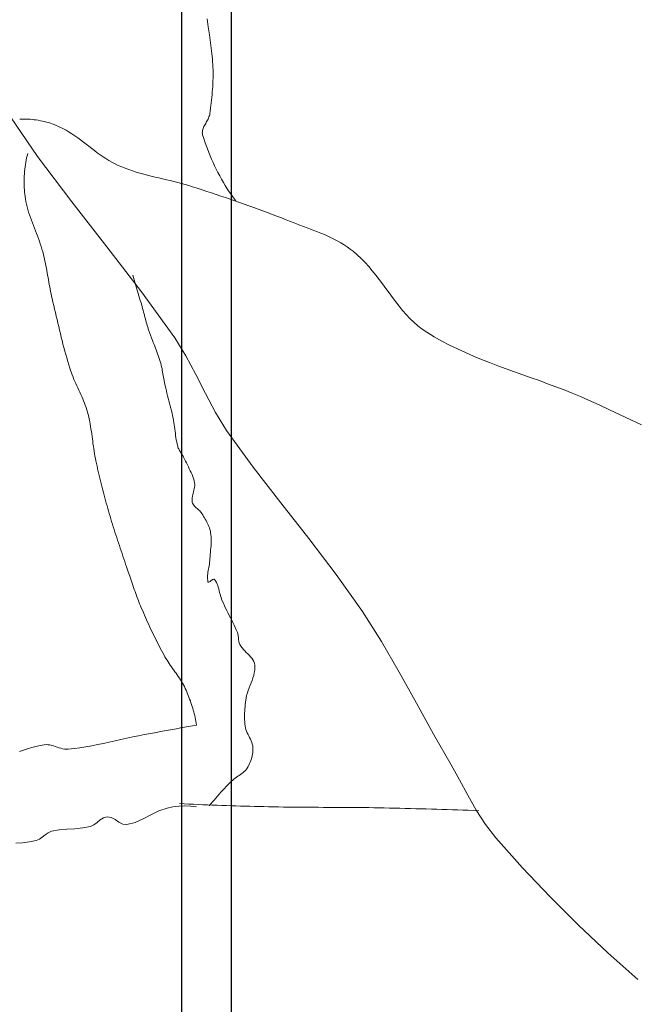
# Model space of a CAD drawing. Units: inches. Extents: x 2656 to 9931, y 1941 to 3068.
# Tile 8 of 46: x 2773 to 2792, y 2502 to 2533. Entities that reach past the tile are written whole.
import ezdxf

# ---------------------------------------------------------------- set-up
doc = ezdxf.new("R2010")
doc.units = ezdxf.units.IN
doc.layers.add('A-ANNO-DIMS', color=2, linetype='Continuous', lineweight=18)
doc.layers.add('A-FURN', color=8, linetype='Continuous', lineweight=13)
doc.styles.get("Standard").update_dxf_attribs({"font": 'arial.ttf'})
doc.dimstyles.new('ISO-25', dxfattribs={"dimtxt": 6, "dimasz": 2.5, "dimexe": 1.25, "dimexo": 0.625, "dimtad": 1, "dimdec": 0, "dimlunit": 3, "dimtxsty": 'Standard', "dimcen": 2.5, "dimadec": 0, "dimazin": 0, "dimtfac": 1, "dimtdec": 0, "dimtmove": 0, "dimatfit": 3, "dimfxl": 1, "dimarcsym": 0})

# ---------------------------------------------------------------- blocks, each defined once
blk = doc.blocks.new('BED-DOUBLE')
for p, q in [((24.978, 30.142), (25.017, 29.893)), ((25.017, 29.893), (25.054, 29.644)), ((25.054, 29.644), (25.087, 29.395)), ((25.087, 29.395), (25.118, 29.145)), ((25.118, 29.145), (25.146, 28.894)), ((25.146, 28.894), (25.153, 28.81)), ((25.153, 28.81), (25.159, 28.725)), ((25.159, 28.725), (25.164, 28.64)), ((25.164, 28.64), (25.166, 28.554)), ((25.166, 28.554), (25.168, 28.469)), ((25.163, 28.213), (25.16, 28.128)), ((25.166, 28.299), (25.163, 28.213)), ((25.168, 28.384), (25.166, 28.299)), ((25.168, 28.469), (25.168, 28.384)), ((25.149, 27.957), (25.142, 27.872)), ((25.155, 28.042), (25.149, 27.957)), ((25.16, 28.128), (25.155, 28.042)), ((25.118, 27.616), (25.108, 27.531)), ((25.127, 27.701), (25.118, 27.616)), ((25.135, 27.787), (25.127, 27.701)), ((25.142, 27.872), (25.135, 27.787)), ((18.699, 27.32), (19.702, 25.863)), ((25.078, 27.276), (25.067, 27.192)), ((25.088, 27.361), (25.078, 27.276)), ((25.098, 27.446), (25.088, 27.361)), ((25.108, 27.531), (25.098, 27.446)), ((19.217, 27.024), (19.153, 27.022)), ((19.28, 27.025), (19.217, 27.024)), ((19.344, 27.025), (19.28, 27.025)), ((19.408, 27.022), (19.344, 27.025)), ((19.472, 27.018), (19.408, 27.022)), ((19.535, 27.013), (19.472, 27.018)), ((19.599, 27.006), (19.535, 27.013)), ((19.663, 26.997), (19.599, 27.006)), ((19.726, 26.987), (19.663, 26.997)), ((19.789, 26.975), (19.726, 26.987)), ((19.852, 26.962), (19.789, 26.975)), ((24.993, 26.99), (24.975, 26.958)), ((25.01, 27.023), (24.993, 26.99)), ((25.026, 27.056), (25.01, 27.023)), ((25.04, 27.09), (25.026, 27.056)), ((25.052, 27.124), (25.04, 27.09)), ((25.061, 27.158), (25.052, 27.124)), ((25.067, 27.192), (25.061, 27.158)), ((19.915, 26.947), (19.852, 26.962)), ((19.977, 26.931), (19.915, 26.947)), ((20.039, 26.914), (19.977, 26.931)), ((20.1, 26.895), (20.039, 26.914)), ((20.16, 26.874), (20.1, 26.895)), ((20.22, 26.852), (20.16, 26.874)), ((20.28, 26.829), (20.22, 26.852)), ((20.338, 26.804), (20.28, 26.829)), ((20.396, 26.778), (20.338, 26.804)), ((20.493, 26.729), (20.396, 26.778)), ((20.588, 26.677), (20.493, 26.729)), ((20.681, 26.622), (20.588, 26.677)), ((24.838, 26.665), (24.833, 26.633)), ((24.845, 26.698), (24.838, 26.665)), ((24.856, 26.73), (24.845, 26.698)), ((24.869, 26.763), (24.856, 26.73)), ((24.884, 26.795), (24.869, 26.763)), ((24.901, 26.827), (24.884, 26.795)), ((24.919, 26.86), (24.901, 26.827)), ((24.937, 26.892), (24.919, 26.86)), ((24.956, 26.925), (24.937, 26.892)), ((24.975, 26.958), (24.956, 26.925)), ((20.773, 26.564), (20.681, 26.622)), ((20.863, 26.503), (20.773, 26.564)), ((20.952, 26.44), (20.863, 26.503)), ((21.04, 26.376), (20.952, 26.44)), ((21.128, 26.31), (21.04, 26.376)), ((24.833, 26.633), (24.832, 26.6)), ((24.832, 26.6), (24.835, 26.567)), ((24.835, 26.567), (24.842, 26.534)), ((24.842, 26.534), (24.876, 26.424)), ((24.876, 26.424), (24.912, 26.314)), ((21.215, 26.244), (21.128, 26.31)), ((21.302, 26.177), (21.215, 26.244)), ((21.389, 26.11), (21.302, 26.177)), ((21.476, 26.044), (21.389, 26.11)), ((21.563, 25.979), (21.476, 26.044)), ((24.912, 26.314), (24.949, 26.205)), ((24.949, 26.205), (24.989, 26.097)), ((24.989, 26.097), (25.031, 25.989)), ((19.348, 25.747), (19.335, 25.677)), ((19.362, 25.817), (19.348, 25.747)), ((19.377, 25.886), (19.362, 25.817)), ((19.394, 25.954), (19.377, 25.886)), ((19.702, 25.863), (20.765, 24.449)), ((21.652, 25.915), (21.563, 25.979)), ((21.741, 25.853), (21.652, 25.915)), ((21.832, 25.793), (21.741, 25.853)), ((21.924, 25.736), (21.832, 25.793)), ((25.031, 25.989), (25.074, 25.882)), ((25.074, 25.882), (25.12, 25.776)), ((25.12, 25.776), (25.167, 25.671)), ((19.306, 25.466), (19.299, 25.395)), ((19.314, 25.537), (19.306, 25.466)), ((19.324, 25.607), (19.314, 25.537)), ((19.335, 25.677), (19.324, 25.607)), ((22.018, 25.682), (21.924, 25.736)), ((22.114, 25.632), (22.018, 25.682)), ((22.211, 25.585), (22.114, 25.632)), ((22.322, 25.537), (22.211, 25.585)), ((22.434, 25.493), (22.322, 25.537)), ((22.547, 25.452), (22.434, 25.493)), ((22.661, 25.413), (22.547, 25.452)), ((25.167, 25.671), (25.216, 25.566)), ((25.216, 25.566), (25.267, 25.462)), ((25.267, 25.462), (25.32, 25.359)), ((19.286, 25.181), (19.285, 25.11)), ((19.289, 25.253), (19.286, 25.181)), ((19.293, 25.324), (19.289, 25.253)), ((19.299, 25.395), (19.293, 25.324)), ((22.775, 25.377), (22.661, 25.413)), ((22.891, 25.343), (22.775, 25.377)), ((23.007, 25.311), (22.891, 25.343)), ((23.124, 25.28), (23.007, 25.311)), ((23.241, 25.25), (23.124, 25.28)), ((23.359, 25.222), (23.241, 25.25)), ((23.476, 25.194), (23.359, 25.222)), ((23.594, 25.166), (23.476, 25.194)), ((23.712, 25.138), (23.594, 25.166)), ((23.83, 25.11), (23.712, 25.138)), ((25.32, 25.359), (25.374, 25.257)), ((25.374, 25.257), (25.431, 25.156)), ((25.431, 25.156), (25.489, 25.056)), ((19.285, 25.11), (19.285, 25.039)), ((19.285, 25.039), (19.287, 24.968)), ((19.287, 24.968), (19.289, 24.897)), ((19.289, 24.897), (19.294, 24.826)), ((19.294, 24.826), (19.3, 24.755)), ((23.948, 25.082), (23.83, 25.11)), ((24.065, 25.053), (23.948, 25.082)), ((24.182, 25.022), (24.065, 25.053)), ((24.299, 24.99), (24.182, 25.022)), ((24.414, 24.956), (24.299, 24.99)), ((24.53, 24.92), (24.414, 24.956)), ((24.676, 24.872), (24.53, 24.92)), ((24.823, 24.824), (24.676, 24.872)), ((24.97, 24.776), (24.823, 24.824)), ((25.489, 25.056), (25.548, 24.957)), ((25.548, 24.957), (25.61, 24.859)), ((25.61, 24.859), (25.673, 24.762)), ((19.3, 24.755), (19.307, 24.684)), ((19.307, 24.684), (19.315, 24.614)), ((19.315, 24.614), (19.325, 24.544)), ((19.325, 24.544), (19.34, 24.459)), ((25.117, 24.728), (24.97, 24.776)), ((25.263, 24.679), (25.117, 24.728)), ((25.41, 24.63), (25.263, 24.679)), ((25.556, 24.581), (25.41, 24.63)), ((25.702, 24.531), (25.556, 24.581)), ((25.673, 24.762), (25.737, 24.667)), ((25.848, 24.481), (25.702, 24.531)), ((25.737, 24.667), (25.804, 24.573)), ((25.804, 24.573), (25.871, 24.48)), ((19.34, 24.459), (19.358, 24.374)), ((19.358, 24.374), (19.378, 24.29)), ((19.378, 24.29), (19.401, 24.206)), ((19.401, 24.206), (19.425, 24.123)), ((20.765, 24.449), (21.855, 23.052)), ((25.994, 24.431), (25.848, 24.481)), ((26.14, 24.38), (25.994, 24.431)), ((26.285, 24.328), (26.14, 24.38)), ((26.431, 24.276), (26.285, 24.328)), ((26.576, 24.223), (26.431, 24.276)), ((26.72, 24.169), (26.576, 24.223)), ((19.425, 24.123), (19.452, 24.04)), ((19.452, 24.04), (19.48, 23.958)), ((19.48, 23.958), (19.509, 23.876)), ((26.865, 24.115), (26.72, 24.169)), ((27.009, 24.06), (26.865, 24.115)), ((27.153, 24.005), (27.009, 24.06)), ((27.297, 23.949), (27.153, 24.005)), ((27.44, 23.891), (27.297, 23.949)), ((19.509, 23.876), (19.54, 23.794)), ((19.54, 23.794), (19.571, 23.713)), ((19.571, 23.713), (19.603, 23.631)), ((19.603, 23.631), (19.635, 23.55)), ((27.548, 23.849), (27.44, 23.891)), ((27.656, 23.807), (27.548, 23.849)), ((27.764, 23.766), (27.656, 23.807)), ((27.873, 23.726), (27.764, 23.766)), ((27.982, 23.685), (27.873, 23.726)), ((28.092, 23.644), (27.982, 23.685)), ((28.201, 23.603), (28.092, 23.644)), ((28.309, 23.561), (28.201, 23.603)), ((19.635, 23.55), (19.666, 23.468)), ((19.666, 23.468), (19.698, 23.387)), ((19.698, 23.387), (19.729, 23.305)), ((19.729, 23.305), (19.758, 23.223)), ((28.418, 23.518), (28.309, 23.561)), ((28.525, 23.474), (28.418, 23.518)), ((28.632, 23.428), (28.525, 23.474)), ((28.738, 23.381), (28.632, 23.428)), ((28.842, 23.332), (28.738, 23.381)), ((28.945, 23.28), (28.842, 23.332)), ((19.758, 23.223), (19.787, 23.141)), ((19.787, 23.141), (19.814, 23.058)), ((19.814, 23.058), (19.84, 22.975)), ((21.855, 23.052), (22.936, 21.65)), ((29.047, 23.227), (28.945, 23.28)), ((29.147, 23.17), (29.047, 23.227)), ((29.245, 23.11), (29.147, 23.17)), ((29.341, 23.048), (29.245, 23.11)), ((29.434, 22.981), (29.341, 23.048)), ((29.526, 22.911), (29.434, 22.981)), ((19.84, 22.975), (19.864, 22.891)), ((19.864, 22.891), (19.882, 22.819)), ((19.882, 22.819), (19.9, 22.747)), ((19.9, 22.747), (19.917, 22.675)), ((19.917, 22.675), (19.932, 22.603)), ((29.656, 22.802), (29.526, 22.911)), ((29.78, 22.685), (29.656, 22.802)), ((29.898, 22.563), (29.78, 22.685)), ((19.932, 22.603), (19.947, 22.53)), ((19.947, 22.53), (19.962, 22.458)), ((19.962, 22.458), (19.976, 22.385)), ((19.976, 22.385), (19.99, 22.312)), ((30.013, 22.435), (29.898, 22.563)), ((30.123, 22.304), (30.013, 22.435)), ((19.99, 22.312), (20.003, 22.239)), ((20.003, 22.239), (20.016, 22.166)), ((20.016, 22.166), (20.029, 22.093)), ((20.029, 22.093), (20.042, 22.02)), ((22.664, 22.169), (22.686, 22.097)), ((22.686, 22.097), (22.708, 22.025)), ((30.231, 22.169), (30.123, 22.304)), ((30.336, 22.032), (30.231, 22.169)), ((20.042, 22.02), (20.055, 21.947)), ((20.055, 21.947), (20.068, 21.874)), ((20.068, 21.874), (20.082, 21.801)), ((20.082, 21.801), (20.095, 21.728)), ((22.708, 22.025), (22.73, 21.953)), ((22.73, 21.953), (22.752, 21.881)), ((22.752, 21.881), (22.774, 21.809)), ((22.774, 21.809), (22.796, 21.737)), ((30.44, 21.893), (30.336, 22.032)), ((30.543, 21.753), (30.44, 21.893)), ((20.095, 21.728), (20.11, 21.655)), ((20.11, 21.655), (20.125, 21.583)), ((20.125, 21.583), (20.14, 21.51)), ((20.14, 21.51), (20.157, 21.438)), ((22.796, 21.737), (22.817, 21.665)), ((22.817, 21.665), (22.839, 21.592)), ((22.839, 21.592), (22.86, 21.52)), ((22.86, 21.52), (22.881, 21.448)), ((22.936, 21.65), (23.974, 20.217)), ((30.646, 21.613), (30.543, 21.753)), ((30.749, 21.474), (30.646, 21.613)), ((30.853, 21.336), (30.749, 21.474)), ((20.157, 21.438), (20.182, 21.329)), ((20.182, 21.329), (20.207, 21.22)), ((20.207, 21.22), (20.232, 21.111)), ((22.881, 21.448), (22.902, 21.376)), ((22.902, 21.376), (22.923, 21.303)), ((22.923, 21.303), (22.944, 21.231)), ((22.944, 21.231), (22.959, 21.179)), ((22.959, 21.179), (22.974, 21.126)), ((30.96, 21.201), (30.853, 21.336)), ((31.069, 21.069), (30.96, 21.201)), ((20.232, 21.111), (20.258, 21.002)), ((20.258, 21.002), (20.283, 20.893)), ((20.283, 20.893), (20.308, 20.784)), ((22.974, 21.126), (22.988, 21.074)), ((22.988, 21.074), (23.003, 21.021)), ((23.003, 21.021), (23.017, 20.968)), ((23.017, 20.968), (23.03, 20.916)), ((23.03, 20.916), (23.044, 20.863)), ((23.044, 20.863), (23.059, 20.81)), ((31.181, 20.941), (31.069, 21.069)), ((31.298, 20.818), (31.181, 20.941)), ((20.308, 20.784), (20.334, 20.675)), ((20.334, 20.675), (20.36, 20.566)), ((20.36, 20.566), (20.386, 20.457)), ((23.059, 20.81), (23.073, 20.758)), ((23.073, 20.758), (23.087, 20.705)), ((23.087, 20.705), (23.102, 20.653)), ((23.102, 20.653), (23.117, 20.601)), ((23.117, 20.601), (23.133, 20.548)), ((23.133, 20.548), (23.142, 20.521)), ((31.419, 20.7), (31.298, 20.818)), ((31.546, 20.59), (31.419, 20.7)), ((31.68, 20.486), (31.546, 20.59)), ((20.386, 20.457), (20.412, 20.349)), ((20.412, 20.349), (20.439, 20.24)), ((20.439, 20.24), (20.467, 20.131)), ((23.142, 20.521), (23.151, 20.493)), ((23.151, 20.493), (23.16, 20.465)), ((23.16, 20.465), (23.17, 20.438)), ((23.17, 20.438), (23.18, 20.41)), ((23.18, 20.41), (23.19, 20.383)), ((23.19, 20.383), (23.2, 20.355)), ((23.2, 20.355), (23.211, 20.328)), ((23.211, 20.328), (23.221, 20.301)), ((23.221, 20.301), (23.231, 20.273)), ((23.231, 20.273), (23.242, 20.246)), ((23.242, 20.246), (23.252, 20.218)), ((31.82, 20.391), (31.68, 20.486)), ((32.053, 20.249), (31.82, 20.391)), ((32.29, 20.116), (32.053, 20.249)), ((20.467, 20.131), (20.494, 20.023)), ((20.494, 20.023), (20.523, 19.915)), ((23.252, 20.218), (23.262, 20.191)), ((23.262, 20.191), (23.283, 20.132)), ((23.283, 20.132), (23.305, 20.073)), ((23.305, 20.073), (23.328, 20.015)), ((23.328, 20.015), (23.35, 19.956)), ((23.35, 19.956), (23.373, 19.898)), ((23.974, 20.217), (24.323, 19.656)), ((32.531, 19.99), (32.29, 20.116)), ((32.775, 19.87), (32.531, 19.99)), ((20.523, 19.915), (20.552, 19.807)), ((20.552, 19.807), (20.581, 19.699)), ((20.581, 19.699), (20.612, 19.591)), ((23.373, 19.898), (23.396, 19.839)), ((23.396, 19.839), (23.418, 19.781)), ((23.418, 19.781), (23.44, 19.722)), ((23.44, 19.722), (23.461, 19.663)), ((23.461, 19.663), (23.482, 19.604)), ((24.323, 19.656), (24.634, 19.073)), ((33.022, 19.757), (32.775, 19.87)), ((33.272, 19.649), (33.022, 19.757)), ((33.525, 19.545), (33.272, 19.649)), ((20.612, 19.591), (20.643, 19.484)), ((20.643, 19.484), (20.675, 19.377)), ((20.675, 19.377), (20.708, 19.27)), ((23.482, 19.604), (23.502, 19.544)), ((23.502, 19.544), (23.521, 19.485)), ((23.521, 19.485), (23.538, 19.425)), ((23.538, 19.425), (23.552, 19.372)), ((23.552, 19.372), (23.565, 19.318)), ((23.565, 19.318), (23.577, 19.265)), ((33.779, 19.445), (33.525, 19.545)), ((34.035, 19.348), (33.779, 19.445)), ((34.292, 19.254), (34.035, 19.348)), ((20.708, 19.27), (20.73, 19.2)), ((20.73, 19.2), (20.755, 19.131)), ((20.755, 19.131), (20.781, 19.062)), ((20.781, 19.062), (20.808, 18.994)), ((23.577, 19.265), (23.587, 19.211)), ((23.587, 19.211), (23.597, 19.157)), ((23.597, 19.157), (23.607, 19.102)), ((23.607, 19.102), (23.616, 19.048)), ((23.616, 19.048), (23.625, 18.994)), ((24.634, 19.073), (24.932, 18.481)), ((34.55, 19.161), (34.292, 19.254)), ((34.809, 19.069), (34.55, 19.161)), ((35.068, 18.977), (34.809, 19.069)), ((20.808, 18.994), (20.836, 18.926)), ((20.836, 18.926), (20.865, 18.859)), ((20.865, 18.859), (20.895, 18.792)), ((20.895, 18.792), (20.925, 18.725)), ((20.925, 18.725), (20.956, 18.658)), ((23.625, 18.994), (23.634, 18.94)), ((23.634, 18.94), (23.643, 18.885)), ((23.643, 18.885), (23.653, 18.831)), ((23.653, 18.831), (23.664, 18.777)), ((23.664, 18.777), (23.675, 18.724)), ((23.675, 18.724), (23.693, 18.646)), ((35.326, 18.885), (35.068, 18.977)), ((35.584, 18.791), (35.326, 18.885)), ((35.841, 18.696), (35.584, 18.791)), ((36.097, 18.598), (35.841, 18.696)), ((20.956, 18.658), (20.987, 18.591)), ((20.987, 18.591), (21.017, 18.524)), ((21.017, 18.524), (21.048, 18.457)), ((21.048, 18.457), (21.078, 18.39)), ((21.078, 18.39), (21.107, 18.322)), ((23.693, 18.646), (23.712, 18.568)), ((23.712, 18.568), (23.732, 18.491)), ((23.732, 18.491), (23.751, 18.414)), ((23.751, 18.414), (23.771, 18.336)), ((24.932, 18.481), (25.243, 17.897)), ((36.351, 18.496), (36.097, 18.598)), ((36.603, 18.391), (36.351, 18.496)), ((36.853, 18.28), (36.603, 18.391)), ((21.107, 18.322), (21.135, 18.255)), ((21.135, 18.255), (21.162, 18.186)), ((21.162, 18.186), (21.188, 18.118)), ((21.188, 18.118), (21.213, 18.049)), ((23.771, 18.336), (23.792, 18.259)), ((23.792, 18.259), (23.812, 18.182)), ((23.812, 18.182), (23.832, 18.105)), ((23.832, 18.105), (23.851, 18.027)), ((37.185, 18.128), (36.853, 18.28)), ((37.515, 17.974), (37.185, 18.128)), ((21.213, 18.049), (21.235, 17.979)), ((21.235, 17.979), (21.256, 17.909)), ((21.256, 17.909), (21.276, 17.834)), ((21.276, 17.834), (21.294, 17.759)), ((23.851, 18.027), (23.87, 17.95)), ((23.87, 17.95), (23.889, 17.872)), ((23.889, 17.872), (23.907, 17.794)), ((23.907, 17.794), (23.923, 17.716)), ((25.243, 17.897), (25.59, 17.336)), ((37.846, 17.819), (37.515, 17.974)), ((38.175, 17.662), (37.846, 17.819)), ((21.294, 17.759), (21.311, 17.684)), ((21.311, 17.684), (21.326, 17.609)), ((21.326, 17.609), (21.34, 17.533)), ((21.34, 17.533), (21.353, 17.457)), ((23.923, 17.716), (23.936, 17.649)), ((23.936, 17.649), (23.948, 17.582)), ((23.948, 17.582), (23.958, 17.515)), ((23.958, 17.515), (23.967, 17.448)), ((38.504, 17.505), (38.175, 17.662)), ((21.353, 17.457), (21.365, 17.38)), ((21.365, 17.38), (21.377, 17.304)), ((21.377, 17.304), (21.387, 17.227)), ((21.387, 17.227), (21.398, 17.151)), ((23.967, 17.448), (23.975, 17.38)), ((23.975, 17.38), (23.984, 17.312)), ((23.984, 17.312), (23.992, 17.245)), ((23.992, 17.245), (24.001, 17.177)), ((24.001, 17.177), (24.011, 17.11)), ((25.59, 17.336), (26.414, 16.194)), ((21.398, 17.151), (21.408, 17.074)), ((21.408, 17.074), (21.418, 16.997)), ((21.418, 16.997), (21.428, 16.92)), ((21.428, 16.92), (21.439, 16.844)), ((24.011, 17.11), (24.022, 17.043)), ((24.022, 17.043), (24.034, 16.976)), ((24.034, 16.976), (24.049, 16.91)), ((24.049, 16.91), (24.065, 16.844)), ((21.439, 16.844), (21.45, 16.767)), ((21.45, 16.767), (21.461, 16.691)), ((21.461, 16.691), (21.473, 16.614)), ((21.473, 16.614), (21.487, 16.538)), ((24.065, 16.844), (24.073, 16.815)), ((24.073, 16.815), (24.084, 16.788)), ((24.084, 16.788), (24.096, 16.761)), ((24.096, 16.761), (24.109, 16.735)), ((24.109, 16.735), (24.124, 16.709)), ((24.124, 16.709), (24.139, 16.684)), ((24.139, 16.684), (24.155, 16.659)), ((24.155, 16.659), (24.171, 16.633)), ((24.171, 16.633), (24.187, 16.608)), ((24.187, 16.608), (24.203, 16.583)), ((24.203, 16.583), (24.218, 16.557)), ((24.218, 16.557), (24.232, 16.531)), ((21.487, 16.538), (21.501, 16.462)), ((21.501, 16.462), (21.516, 16.386)), ((21.516, 16.386), (21.534, 16.304)), ((21.534, 16.304), (21.553, 16.221)), ((24.232, 16.531), (24.245, 16.504)), ((24.245, 16.504), (24.274, 16.444)), ((24.274, 16.444), (24.304, 16.384)), ((24.304, 16.384), (24.335, 16.323)), ((24.335, 16.323), (24.366, 16.264)), ((24.366, 16.264), (24.397, 16.203)), ((21.553, 16.221), (21.571, 16.139)), ((21.571, 16.139), (21.59, 16.056)), ((21.59, 16.056), (21.609, 15.974)), ((21.609, 15.974), (21.629, 15.892)), ((24.397, 16.203), (24.427, 16.143)), ((24.427, 16.143), (24.457, 16.083)), ((24.457, 16.083), (24.485, 16.022)), ((24.485, 16.022), (24.512, 15.96)), ((24.512, 15.96), (24.536, 15.898)), ((26.414, 16.194), (27.275, 15.078)), ((21.629, 15.892), (21.649, 15.809)), ((21.649, 15.809), (21.669, 15.727)), ((21.669, 15.727), (21.69, 15.645)), ((21.69, 15.645), (21.711, 15.563)), ((24.536, 15.898), (24.558, 15.835)), ((24.558, 15.835), (24.576, 15.771)), ((24.576, 15.771), (24.591, 15.705)), ((24.591, 15.705), (24.596, 15.659)), ((24.596, 15.659), (24.596, 15.613)), ((21.711, 15.563), (21.732, 15.481)), ((21.732, 15.481), (21.753, 15.4)), ((21.753, 15.4), (21.775, 15.318)), ((24.533, 15.333), (24.522, 15.287)), ((24.545, 15.38), (24.533, 15.333)), ((24.559, 15.427), (24.545, 15.38)), ((24.571, 15.473), (24.559, 15.427)), ((24.583, 15.52), (24.571, 15.473)), ((24.591, 15.567), (24.583, 15.52)), ((24.596, 15.613), (24.591, 15.567)), ((21.775, 15.318), (21.797, 15.236)), ((21.797, 15.236), (21.819, 15.154)), ((21.819, 15.154), (21.842, 15.073)), ((21.842, 15.073), (21.865, 14.991)), ((24.515, 15.24), (24.511, 15.194)), ((24.511, 15.194), (24.512, 15.148)), ((24.512, 15.148), (24.519, 15.103)), ((24.522, 15.287), (24.515, 15.24)), ((24.519, 15.103), (24.53, 15.069)), ((24.53, 15.069), (24.546, 15.038)), ((24.546, 15.038), (24.565, 15.009)), ((27.275, 15.078), (28.146, 13.969)), ((21.865, 14.991), (21.888, 14.91)), ((21.888, 14.91), (21.911, 14.829)), ((21.911, 14.829), (21.934, 14.748)), ((21.934, 14.748), (21.959, 14.664)), ((24.565, 15.009), (24.588, 14.982)), ((24.588, 14.982), (24.613, 14.956)), ((24.613, 14.956), (24.639, 14.931)), ((24.639, 14.931), (24.667, 14.907)), ((24.667, 14.907), (24.696, 14.882)), ((24.696, 14.882), (24.724, 14.858)), ((24.724, 14.858), (24.751, 14.833)), ((24.751, 14.833), (24.777, 14.806)), ((24.777, 14.806), (24.8, 14.779)), ((24.8, 14.779), (24.82, 14.749)), ((24.82, 14.749), (24.846, 14.706)), ((21.959, 14.664), (21.984, 14.581)), ((21.984, 14.581), (22.009, 14.498)), ((22.009, 14.498), (22.034, 14.415)), ((22.034, 14.415), (22.06, 14.332)), ((24.846, 14.706), (24.873, 14.662)), ((24.873, 14.662), (24.899, 14.619)), ((24.899, 14.619), (24.924, 14.575)), ((24.924, 14.575), (24.949, 14.53)), ((24.949, 14.53), (24.974, 14.485)), ((24.974, 14.485), (24.996, 14.44)), ((24.996, 14.44), (25.018, 14.394)), ((22.06, 14.332), (22.086, 14.249)), ((22.086, 14.249), (22.113, 14.166)), ((22.113, 14.166), (22.14, 14.083)), ((25.018, 14.394), (25.037, 14.347)), ((25.037, 14.347), (25.055, 14.3)), ((25.055, 14.3), (25.07, 14.252)), ((25.07, 14.252), (25.083, 14.204)), ((25.083, 14.204), (25.092, 14.155)), ((25.092, 14.155), (25.101, 14.088)), ((22.14, 14.083), (22.167, 14.001)), ((22.167, 14.001), (22.194, 13.918)), ((22.194, 13.918), (22.221, 13.835)), ((22.221, 13.835), (22.249, 13.753)), ((25.101, 14.088), (25.107, 14.021)), ((25.107, 13.819), (25.103, 13.751)), ((25.107, 14.021), (25.11, 13.954)), ((25.11, 13.886), (25.107, 13.819)), ((25.11, 13.954), (25.11, 13.886)), ((28.146, 13.969), (29.001, 12.85)), ((22.249, 13.753), (22.277, 13.671)), ((22.277, 13.671), (22.304, 13.588)), ((22.304, 13.588), (22.332, 13.506)), ((22.332, 13.506), (22.36, 13.424)), ((25.085, 13.548), (25.078, 13.48)), ((25.092, 13.616), (25.085, 13.548)), ((25.098, 13.684), (25.092, 13.616)), ((25.103, 13.751), (25.098, 13.684)), ((22.36, 13.424), (22.388, 13.341)), ((22.388, 13.341), (22.417, 13.259)), ((22.417, 13.259), (22.445, 13.177)), ((22.445, 13.177), (22.473, 13.094)), ((25.051, 13.177), (25.043, 13.126)), ((25.058, 13.227), (25.051, 13.177)), ((25.062, 13.278), (25.058, 13.227)), ((25.066, 13.345), (25.062, 13.278)), ((25.072, 13.413), (25.066, 13.345)), ((25.078, 13.48), (25.072, 13.413)), ((22.473, 13.094), (22.495, 13.03)), ((22.495, 13.03), (22.516, 12.966)), ((22.516, 12.966), (22.538, 12.901)), ((22.538, 12.901), (22.56, 12.837)), ((24.999, 12.872), (24.994, 12.822)), ((25.006, 12.923), (24.999, 12.872)), ((25.015, 12.973), (25.006, 12.923)), ((25.024, 13.024), (25.015, 12.973)), ((25.034, 13.075), (25.024, 13.024)), ((25.043, 13.126), (25.034, 13.075)), ((22.56, 12.837), (22.581, 12.773)), ((22.581, 12.773), (22.603, 12.708)), ((22.603, 12.708), (22.625, 12.644)), ((22.625, 12.644), (22.647, 12.58)), ((22.647, 12.58), (22.669, 12.516)), ((24.994, 12.822), (24.992, 12.772)), ((24.992, 12.772), (24.994, 12.722)), ((24.994, 12.722), (24.999, 12.673)), ((24.999, 12.673), (25.009, 12.624)), ((25.009, 12.624), (25.016, 12.612)), ((25.016, 12.612), (25.026, 12.609)), ((25.026, 12.609), (25.039, 12.612)), ((25.039, 12.612), (25.055, 12.621)), ((25.055, 12.621), (25.073, 12.633)), ((25.073, 12.633), (25.092, 12.648)), ((25.092, 12.648), (25.112, 12.664)), ((25.112, 12.664), (25.132, 12.679)), ((25.132, 12.679), (25.152, 12.693)), ((25.152, 12.693), (25.17, 12.702)), ((25.17, 12.702), (25.187, 12.708)), ((25.187, 12.708), (25.202, 12.706)), ((25.202, 12.706), (25.214, 12.697)), ((25.214, 12.697), (25.244, 12.653)), ((25.244, 12.653), (25.27, 12.606)), ((25.27, 12.606), (25.292, 12.557)), ((29.001, 12.85), (29.816, 11.701)), ((22.669, 12.516), (22.692, 12.451)), ((22.692, 12.451), (22.714, 12.387)), ((22.714, 12.387), (22.737, 12.324)), ((22.737, 12.324), (22.76, 12.26)), ((22.76, 12.26), (22.784, 12.196)), ((25.292, 12.557), (25.312, 12.507)), ((25.312, 12.507), (25.329, 12.455)), ((25.329, 12.455), (25.344, 12.402)), ((25.344, 12.402), (25.358, 12.349)), ((25.358, 12.349), (25.372, 12.295)), ((25.372, 12.295), (25.386, 12.242)), ((22.784, 12.196), (22.807, 12.132)), ((22.807, 12.132), (22.832, 12.069)), ((22.832, 12.069), (22.856, 12.006)), ((22.856, 12.006), (22.881, 11.943)), ((25.386, 12.242), (25.4, 12.188)), ((25.4, 12.188), (25.416, 12.136)), ((25.416, 12.136), (25.433, 12.084)), ((25.433, 12.084), (25.453, 12.033)), ((25.453, 12.033), (25.487, 11.956)), ((25.487, 11.956), (25.522, 11.88)), ((22.881, 11.943), (22.907, 11.88)), ((22.907, 11.88), (22.933, 11.817)), ((22.933, 11.817), (22.965, 11.742)), ((22.965, 11.742), (22.998, 11.667)), ((22.998, 11.667), (23.03, 11.592)), ((25.522, 11.88), (25.559, 11.805)), ((25.559, 11.805), (25.596, 11.729)), ((25.596, 11.729), (25.634, 11.654)), ((25.634, 11.654), (25.672, 11.579)), ((29.816, 11.701), (30.407, 10.77)), ((23.03, 11.592), (23.063, 11.517)), ((23.063, 11.517), (23.097, 11.442)), ((23.097, 11.442), (23.13, 11.367)), ((23.13, 11.367), (23.164, 11.293)), ((25.672, 11.579), (25.71, 11.505)), ((25.71, 11.505), (25.748, 11.43)), ((25.748, 11.43), (25.786, 11.354)), ((25.786, 11.354), (25.822, 11.279)), ((23.164, 11.293), (23.198, 11.218)), ((23.198, 11.218), (23.233, 11.144)), ((23.233, 11.144), (23.268, 11.07)), ((23.268, 11.07), (23.303, 10.996)), ((25.822, 11.279), (25.857, 11.203)), ((25.857, 11.203), (25.891, 11.126)), ((25.891, 11.126), (25.924, 11.048)), ((25.924, 11.048), (25.933, 11.021)), ((23.303, 10.996), (23.339, 10.922)), ((23.339, 10.922), (23.375, 10.849)), ((23.375, 10.849), (23.412, 10.775)), ((23.412, 10.775), (23.449, 10.702)), ((25.933, 11.021), (25.941, 10.992)), ((25.941, 10.992), (25.946, 10.963)), ((25.946, 10.963), (25.951, 10.933)), ((25.951, 10.933), (25.954, 10.903)), ((25.954, 10.903), (25.957, 10.873)), ((25.957, 10.873), (25.959, 10.843)), ((25.959, 10.843), (25.963, 10.813)), ((25.963, 10.813), (25.967, 10.784)), ((25.967, 10.784), (25.972, 10.755)), ((25.972, 10.755), (25.98, 10.727)), ((25.98, 10.727), (25.989, 10.699)), ((30.407, 10.77), (30.961, 9.816)), ((23.449, 10.702), (23.486, 10.629)), ((23.486, 10.629), (23.524, 10.557)), ((23.524, 10.557), (23.562, 10.484)), ((23.562, 10.484), (23.6, 10.412)), ((25.989, 10.699), (26.002, 10.672)), ((26.002, 10.672), (26.033, 10.62)), ((26.033, 10.62), (26.07, 10.57)), ((26.07, 10.57), (26.111, 10.522)), ((26.111, 10.522), (26.155, 10.476)), ((26.155, 10.476), (26.2, 10.43)), ((26.2, 10.43), (26.245, 10.385)), ((23.6, 10.412), (23.639, 10.34)), ((23.639, 10.34), (23.669, 10.287)), ((23.669, 10.287), (23.7, 10.234)), ((23.7, 10.234), (23.733, 10.182)), ((23.733, 10.182), (23.766, 10.131)), ((23.766, 10.131), (23.8, 10.08)), ((26.245, 10.385), (26.289, 10.34)), ((26.289, 10.34), (26.332, 10.293)), ((26.332, 10.293), (26.37, 10.246)), ((26.37, 10.246), (26.404, 10.196)), ((26.404, 10.196), (26.432, 10.144)), ((26.432, 10.144), (26.452, 10.089)), ((23.8, 10.08), (23.835, 10.029)), ((23.835, 10.029), (23.871, 9.979)), ((23.871, 9.979), (23.906, 9.928)), ((23.906, 9.928), (23.942, 9.878)), ((23.942, 9.878), (23.978, 9.828)), ((23.978, 9.828), (24.014, 9.778)), ((26.464, 9.871), (26.451, 9.793)), ((26.452, 10.089), (26.464, 10.031)), ((26.464, 10.031), (26.468, 9.951)), ((26.468, 9.951), (26.464, 9.871)), ((30.961, 9.816), (31.497, 8.85)), ((24.014, 9.778), (24.049, 9.728)), ((24.049, 9.728), (24.084, 9.677)), ((24.084, 9.677), (24.118, 9.627)), ((24.118, 9.627), (24.151, 9.575)), ((24.151, 9.575), (24.184, 9.523)), ((24.184, 9.523), (24.215, 9.471)), ((26.381, 9.559), (26.351, 9.481)), ((26.408, 9.637), (26.381, 9.559)), ((26.432, 9.714), (26.408, 9.637)), ((26.451, 9.793), (26.432, 9.714)), ((24.215, 9.471), (24.245, 9.417)), ((24.245, 9.417), (24.273, 9.363)), ((24.273, 9.363), (24.3, 9.308)), ((24.3, 9.308), (24.325, 9.254)), ((24.325, 9.254), (24.349, 9.199)), ((24.349, 9.199), (24.372, 9.144)), ((26.26, 9.248), (26.234, 9.17)), ((26.289, 9.326), (26.26, 9.248)), ((26.32, 9.404), (26.289, 9.326)), ((26.351, 9.481), (26.32, 9.404)), ((24.372, 9.144), (24.395, 9.088)), ((24.395, 9.088), (24.417, 9.033)), ((24.417, 9.033), (24.438, 8.977)), ((24.438, 8.977), (24.459, 8.92)), ((24.459, 8.92), (24.479, 8.863)), ((26.187, 8.944), (26.177, 8.877)), ((26.197, 9.011), (26.187, 8.944)), ((26.212, 9.091), (26.197, 9.011)), ((26.234, 9.17), (26.212, 9.091)), ((24.479, 8.863), (24.497, 8.806)), ((24.497, 8.806), (24.516, 8.749)), ((24.516, 8.749), (24.533, 8.692)), ((24.533, 8.692), (24.55, 8.634)), ((24.55, 8.634), (24.566, 8.576)), ((26.152, 8.607), (26.148, 8.539)), ((26.156, 8.674), (26.152, 8.607)), ((26.162, 8.742), (26.156, 8.674)), ((26.169, 8.81), (26.162, 8.742)), ((26.177, 8.877), (26.169, 8.81)), ((31.497, 8.85), (32.03, 7.883)), ((24.566, 8.576), (24.581, 8.518)), ((24.581, 8.518), (24.595, 8.46)), ((24.595, 8.46), (24.608, 8.401)), ((24.608, 8.401), (24.621, 8.342)), ((24.621, 8.342), (24.633, 8.284)), ((24.633, 8.284), (24.644, 8.225)), ((26.148, 8.539), (26.147, 8.471)), ((26.147, 8.471), (26.147, 8.403)), ((26.147, 8.403), (26.149, 8.336)), ((26.149, 8.336), (26.153, 8.268)), ((23.654, 7.985), (23.529, 7.962)), ((23.779, 8.008), (23.654, 7.985)), ((23.904, 8.031), (23.779, 8.008)), ((24.029, 8.053), (23.904, 8.031)), ((24.154, 8.076), (24.029, 8.053)), ((24.279, 8.099), (24.154, 8.076)), ((24.404, 8.121), (24.279, 8.099)), ((24.529, 8.144), (24.404, 8.121)), ((24.654, 8.166), (24.529, 8.144)), ((24.644, 8.225), (24.654, 8.166)), ((26.153, 8.268), (26.158, 8.201)), ((26.158, 8.201), (26.166, 8.134)), ((26.166, 8.134), (26.177, 8.081)), ((26.177, 8.081), (26.191, 8.029)), ((26.191, 8.029), (26.21, 7.978)), ((26.21, 7.978), (26.232, 7.927)), ((22.118, 7.677), (21.936, 7.637)), ((22.3, 7.717), (22.118, 7.677)), ((22.482, 7.757), (22.3, 7.717)), ((22.664, 7.796), (22.482, 7.757)), ((22.847, 7.833), (22.664, 7.796)), ((23.029, 7.869), (22.847, 7.833)), ((23.154, 7.892), (23.029, 7.869)), ((23.279, 7.915), (23.154, 7.892)), ((23.404, 7.939), (23.279, 7.915)), ((23.529, 7.962), (23.404, 7.939)), ((26.232, 7.927), (26.256, 7.877)), ((26.256, 7.877), (26.281, 7.828)), ((26.281, 7.828), (26.306, 7.778)), ((26.306, 7.778), (26.33, 7.728)), ((26.33, 7.728), (26.353, 7.678)), ((26.353, 7.678), (26.373, 7.627)), ((32.03, 7.883), (32.577, 6.925)), ((19.264, 7.386), (19.137, 7.343)), ((19.392, 7.427), (19.264, 7.386)), ((19.52, 7.464), (19.392, 7.427)), ((19.649, 7.498), (19.52, 7.464)), ((19.779, 7.528), (19.649, 7.498)), ((19.911, 7.552), (19.779, 7.528)), ((19.968, 7.558), (19.911, 7.552)), ((20.025, 7.556), (19.968, 7.558)), ((20.082, 7.548), (20.025, 7.556)), ((20.139, 7.535), (20.082, 7.548)), ((20.196, 7.519), (20.139, 7.535)), ((20.252, 7.5), (20.196, 7.519)), ((20.309, 7.48), (20.252, 7.5)), ((20.366, 7.461), (20.309, 7.48)), ((20.423, 7.444), (20.366, 7.461)), ((20.48, 7.429), (20.423, 7.444)), ((20.538, 7.419), (20.48, 7.429)), ((20.595, 7.414), (20.538, 7.419)), ((20.653, 7.416), (20.595, 7.414)), ((20.837, 7.437), (20.653, 7.416)), ((21.022, 7.463), (20.837, 7.437)), ((21.205, 7.492), (21.022, 7.463)), ((21.388, 7.525), (21.205, 7.492)), ((21.571, 7.56), (21.388, 7.525)), ((21.754, 7.598), (21.571, 7.56)), ((21.936, 7.637), (21.754, 7.598)), ((26.373, 7.627), (26.389, 7.576)), ((26.389, 7.576), (26.4, 7.524)), ((26.4, 7.524), (26.406, 7.47)), ((26.406, 7.367), (26.402, 7.316)), ((26.406, 7.47), (26.407, 7.419)), ((26.407, 7.419), (26.406, 7.367)), ((26.344, 7.063), (26.326, 7.014)), ((26.36, 7.112), (26.344, 7.063)), ((26.374, 7.163), (26.36, 7.112)), ((26.386, 7.213), (26.374, 7.163)), ((26.395, 7.265), (26.386, 7.213)), ((26.402, 7.316), (26.395, 7.265)), ((26.173, 6.754), (26.139, 6.72)), ((26.205, 6.791), (26.173, 6.754)), ((26.233, 6.83), (26.205, 6.791)), ((26.259, 6.874), (26.233, 6.83)), ((26.283, 6.919), (26.259, 6.874)), ((26.306, 6.966), (26.283, 6.919)), ((26.326, 7.014), (26.306, 6.966)), ((32.577, 6.925), (32.84, 6.459)), ((25.78, 6.456), (25.744, 6.423)), ((25.818, 6.488), (25.78, 6.456)), ((25.858, 6.517), (25.818, 6.488)), ((25.899, 6.546), (25.858, 6.517)), ((25.94, 6.574), (25.899, 6.546)), ((25.982, 6.601), (25.94, 6.574)), ((26.023, 6.63), (25.982, 6.601)), ((26.063, 6.658), (26.023, 6.63)), ((26.102, 6.688), (26.063, 6.658)), ((26.139, 6.72), (26.102, 6.688)), ((32.84, 6.459), (33.095, 5.989)), ((25.465, 6.135), (25.41, 6.076)), ((25.52, 6.193), (25.465, 6.135)), ((25.575, 6.251), (25.52, 6.193)), ((25.631, 6.309), (25.575, 6.251)), ((25.687, 6.366), (25.631, 6.309)), ((25.744, 6.423), (25.687, 6.366)), ((25.197, 5.835), (25.144, 5.774)), ((25.249, 5.896), (25.197, 5.835)), ((25.302, 5.956), (25.249, 5.896)), ((25.356, 6.016), (25.302, 5.956)), ((25.41, 6.076), (25.356, 6.016)), ((33.095, 5.989), (33.36, 5.524)), ((23.738, 5.584), (23.481, 5.494)), ((23.917, 5.622), (23.738, 5.584)), ((24.099, 5.644), (23.917, 5.622)), ((24.282, 5.652), (24.099, 5.644)), ((24.267, 5.715), (24.121, 5.722)), ((24.413, 5.709), (24.267, 5.715)), ((24.466, 5.645), (24.282, 5.652)), ((24.559, 5.702), (24.413, 5.709)), ((24.647, 5.623), (24.466, 5.645)), ((24.705, 5.696), (24.559, 5.702)), ((24.851, 5.69), (24.705, 5.696)), ((24.997, 5.684), (24.851, 5.69)), ((25.143, 5.678), (24.997, 5.684)), ((25.093, 5.712), (25.042, 5.65)), ((25.144, 5.774), (25.093, 5.712)), ((25.29, 5.673), (25.143, 5.678)), ((25.436, 5.667), (25.29, 5.673)), ((25.582, 5.662), (25.436, 5.667)), ((25.728, 5.657), (25.582, 5.662)), ((25.874, 5.653), (25.728, 5.657)), ((26.02, 5.648), (25.874, 5.653)), ((26.166, 5.644), (26.02, 5.648)), ((26.313, 5.64), (26.166, 5.644)), ((26.459, 5.636), (26.313, 5.64)), ((26.605, 5.632), (26.459, 5.636)), ((26.751, 5.628), (26.605, 5.632)), ((26.897, 5.625), (26.751, 5.628)), ((27.044, 5.622), (26.897, 5.625)), ((27.2, 5.619), (27.044, 5.622)), ((27.356, 5.616), (27.2, 5.619)), ((27.513, 5.614), (27.356, 5.616)), ((27.669, 5.612), (27.513, 5.614)), ((27.825, 5.611), (27.669, 5.612)), ((27.982, 5.61), (27.825, 5.611)), ((28.138, 5.609), (27.982, 5.61)), ((28.294, 5.608), (28.138, 5.609)), ((28.451, 5.608), (28.294, 5.608)), ((28.607, 5.607), (28.451, 5.608)), ((28.763, 5.607), (28.607, 5.607)), ((28.92, 5.606), (28.763, 5.607)), ((29.076, 5.606), (28.92, 5.606)), ((29.232, 5.605), (29.076, 5.606)), ((29.389, 5.604), (29.232, 5.605)), ((29.545, 5.603), (29.389, 5.604)), ((29.702, 5.601), (29.545, 5.603)), ((29.858, 5.6), (29.702, 5.601)), ((30.014, 5.597), (29.858, 5.6)), ((30.171, 5.595), (30.014, 5.597)), ((30.334, 5.592), (30.171, 5.595)), ((30.497, 5.588), (30.334, 5.592)), ((30.661, 5.585), (30.497, 5.588)), ((30.824, 5.581), (30.661, 5.585)), ((30.987, 5.578), (30.824, 5.581)), ((31.151, 5.574), (30.987, 5.578)), ((31.314, 5.57), (31.151, 5.574)), ((31.477, 5.565), (31.314, 5.57)), ((31.64, 5.561), (31.477, 5.565)), ((31.804, 5.556), (31.64, 5.561)), ((31.967, 5.552), (31.804, 5.556)), ((32.13, 5.547), (31.967, 5.552)), ((32.294, 5.542), (32.13, 5.547)), ((32.457, 5.537), (32.294, 5.542)), ((32.62, 5.531), (32.457, 5.537)), ((32.784, 5.526), (32.62, 5.531)), ((32.947, 5.52), (32.784, 5.526)), ((33.11, 5.515), (32.947, 5.52)), ((33.36, 5.524), (33.647, 5.076)), ((21.656, 5.218), (21.558, 5.137)), ((21.758, 5.284), (21.656, 5.218)), ((21.872, 5.315), (21.758, 5.284)), ((21.998, 5.292), (21.872, 5.315)), ((22.118, 5.226), (21.998, 5.292)), ((22.235, 5.148), (22.118, 5.226)), ((22.989, 5.248), (22.74, 5.14)), ((23.234, 5.374), (22.989, 5.248)), ((23.481, 5.494), (23.234, 5.374)), ((33.273, 5.509), (33.11, 5.515)), ((33.437, 5.503), (33.273, 5.509)), ((20.371, 4.906), (20.131, 4.861)), ((20.616, 4.928), (20.371, 4.906)), ((20.862, 4.943), (20.616, 4.928)), ((21.107, 4.965), (20.862, 4.943)), ((21.347, 5.011), (21.107, 4.965)), ((21.457, 5.061), (21.347, 5.011)), ((21.558, 5.137), (21.457, 5.061)), ((22.354, 5.087), (22.235, 5.148)), ((22.479, 5.073), (22.354, 5.087)), ((22.74, 5.14), (22.479, 5.073)), ((33.647, 5.076), (33.973, 4.657)), ((19.758, 4.617), (19.657, 4.574)), ((19.85, 4.681), (19.758, 4.617)), ((19.938, 4.753), (19.85, 4.681)), ((20.03, 4.818), (19.938, 4.753)), ((20.131, 4.861), (20.03, 4.818)), ((33.973, 4.657), (34.806, 3.726)), ((19.236, 4.507), (19.022, 4.492)), ((19.448, 4.533), (19.236, 4.507)), ((19.657, 4.574), (19.448, 4.533)), ((34.806, 3.726), (35.666, 2.819)), ((35.666, 2.819), (36.55, 1.936)), ((36.55, 1.936), (37.459, 1.078)), ((37.459, 1.078), (38.392, 0.247))]:
    blk.add_line(p, q)
blk = doc.blocks.new('*D31')
at = {"layer": 'A-ANNO-DIMS', "color": 0, "lineweight": -2, "transparency": 16777216}
for p, q in [((2753.358, 2502.145), (2753.358, 2488.227)), ((2841.982, 2502.145), (2841.982, 2488.227)), ((2755.858, 2489.477), (2839.482, 2489.477)), ((2841.982, 2489.477), (2952.348, 2489.477))]:
    blk.add_line(p, q, dxfattribs=at)
at = {"layer": 'A-ANNO-DIMS', "color": 0, "transparency": 16777216}
for points in [[(2755.858, 2489.893), (2755.858, 2489.06), (2753.358, 2489.477)], [(2839.482, 2489.893), (2839.482, 2489.06), (2841.982, 2489.477)]]:
    blk.add_solid(points, dxfattribs=at)
at = {"layer": 'Defpoints', "color": 0, "transparency": 16777216}
for p in [(2753.358, 2502.77), (2841.982, 2502.77), (2841.982, 2489.477)]:
    blk.add_point(p, dxfattribs=at)
at = {"layer": 'A-ANNO-DIMS', "color": 0, "transparency": 16777216, "insert": (2898.415, 2493.206), "char_height": 6, "attachment_point": 5}
blk.add_mtext('DOUBLE BED 7\'-4 1/2" TYP.', dxfattribs=at)
blk = doc.blocks.new('*D113')
at = {"layer": 'A-ANNO-DIMS', "color": 0, "lineweight": -2, "transparency": 16777216}
for p, q in [((2752.157, 2300.725), (2752.157, 2674.45)), ((2809.769, 2300.725), (2809.769, 2674.45)), ((2754.657, 2673.2), (2807.269, 2673.2))]:
    blk.add_line(p, q, dxfattribs=at)
at = {"layer": 'A-ANNO-DIMS', "color": 0, "transparency": 16777216}
for points in [[(2754.657, 2673.617), (2754.657, 2672.784), (2752.157, 2673.2)], [(2807.269, 2673.617), (2807.269, 2672.784), (2809.769, 2673.2)]]:
    blk.add_solid(points, dxfattribs=at)
at = {"layer": 'Defpoints', "color": 0, "transparency": 16777216}
for p in [(2809.769, 2673.2), (2752.157, 2300.1), (2809.769, 2300.1)]:
    blk.add_point(p, dxfattribs=at)
at = {"layer": 'A-ANNO-DIMS', "color": 0, "transparency": 16777216, "insert": (2780.963, 2676.928), "char_height": 6, "attachment_point": 5}
blk.add_mtext('4\'-9 1/2"', dxfattribs=at)
blk = doc.blocks.new('*D129')
at = {"layer": 'A-ANNO-DIMS', "color": 0, "lineweight": -2, "transparency": 16777216}
for p, q in [((2752.157, 2601.146), (2752.157, 2009.273)), ((2777.587, 2557.74), (2777.587, 2009.273)), ((2754.657, 2010.523), (2775.087, 2010.523)), ((2777.587, 2010.523), (2811.37, 2010.523))]:
    blk.add_line(p, q, dxfattribs=at)
at = {"layer": 'A-ANNO-DIMS', "color": 0, "transparency": 16777216}
for points in [[(2754.657, 2010.939), (2754.657, 2010.106), (2752.157, 2010.523)], [(2775.087, 2010.939), (2775.087, 2010.106), (2777.587, 2010.523)]]:
    blk.add_solid(points, dxfattribs=at)
at = {"layer": 'Defpoints', "color": 0, "transparency": 16777216}
for p in [(2752.157, 2601.771), (2777.587, 2558.365), (2777.587, 2010.523)]:
    blk.add_point(p, dxfattribs=at)
at = {"layer": 'A-ANNO-DIMS', "color": 0, "transparency": 16777216, "insert": (2795.728, 2014.25), "char_height": 6, "attachment_point": 5}
blk.add_mtext('2\'-1 1/2"', dxfattribs=at)
blk = doc.blocks.new('*D132')
at = {"layer": 'A-ANNO-DIMS', "color": 0, "lineweight": -2, "transparency": 16777216}
for p, q in [((2763.467, 2366.557), (2763.467, 2674.45)), ((2805.965, 2366.557), (2805.965, 2674.45)), ((2765.967, 2673.2), (2803.465, 2673.2))]:
    blk.add_line(p, q, dxfattribs=at)
at = {"layer": 'A-ANNO-DIMS', "color": 0, "transparency": 16777216}
for points in [[(2765.967, 2673.617), (2765.967, 2672.784), (2763.467, 2673.2)], [(2803.465, 2673.617), (2803.465, 2672.784), (2805.965, 2673.2)]]:
    blk.add_solid(points, dxfattribs=at)
at = {"layer": 'Defpoints', "color": 0, "transparency": 16777216}
for p in [(2805.965, 2673.2), (2763.467, 2365.932), (2805.965, 2365.932)]:
    blk.add_point(p, dxfattribs=at)
at = {"layer": 'A-ANNO-DIMS', "color": 0, "transparency": 16777216, "insert": (2784.716, 2676.93), "char_height": 6, "attachment_point": 5}
blk.add_mtext('3\'-6 1/2"', dxfattribs=at)
blk = doc.blocks.new('*D134')
at = {"layer": 'A-ANNO-DIMS', "color": 0, "lineweight": -2, "transparency": 16777216}
for p, q in [((2752.157, 2300.725), (2752.157, 2674.45)), ((2763.467, 2347.433), (2763.467, 2674.45)), ((2754.657, 2673.2), (2760.967, 2673.2)), ((2763.467, 2673.2), (2801.809, 2673.2))]:
    blk.add_line(p, q, dxfattribs=at)
at = {"layer": 'A-ANNO-DIMS', "color": 0, "transparency": 16777216}
for points in [[(2754.657, 2673.617), (2754.657, 2672.784), (2752.157, 2673.2)], [(2760.967, 2673.617), (2760.967, 2672.784), (2763.467, 2673.2)]]:
    blk.add_solid(points, dxfattribs=at)
at = {"layer": 'Defpoints', "color": 0, "transparency": 16777216}
for p in [(2763.467, 2673.2), (2763.467, 2346.808), (2752.157, 2300.1)]:
    blk.add_point(p, dxfattribs=at)
at = {"layer": 'A-ANNO-DIMS', "color": 0, "transparency": 16777216, "insert": (2783.888, 2676.928), "char_height": 6, "attachment_point": 5}
blk.add_mtext('0\'-11 1/2"', dxfattribs=at)
blk = doc.blocks.new('*D136')
at = {"layer": 'A-ANNO-DIMS', "color": 0, "lineweight": -2, "transparency": 16777216}
for p, q in [((2765.357, 2375.042), (2765.357, 2674.45)), ((2779.142, 2375.042), (2779.142, 2674.45)), ((2767.857, 2673.2), (2776.642, 2673.2)), ((2779.142, 2673.2), (2798.277, 2673.2))]:
    blk.add_line(p, q, dxfattribs=at)
at = {"layer": 'A-ANNO-DIMS', "color": 0, "transparency": 16777216}
for points in [[(2767.857, 2673.617), (2767.857, 2672.784), (2765.357, 2673.2)], [(2776.642, 2673.617), (2776.642, 2672.784), (2779.142, 2673.2)]]:
    blk.add_solid(points, dxfattribs=at)
at = {"layer": 'Defpoints', "color": 0, "transparency": 16777216}
for p in [(2779.142, 2673.2), (2765.357, 2374.417), (2779.142, 2374.417)]:
    blk.add_point(p, dxfattribs=at)
at = {"layer": 'A-ANNO-DIMS', "color": 0, "transparency": 16777216, "insert": (2789.959, 2676.838), "char_height": 6, "attachment_point": 5}
blk.add_mtext('1\'-2"', dxfattribs=at)
blk = doc.blocks.new('*D137')
at = {"layer": 'A-ANNO-DIMS', "color": 0, "lineweight": -2, "transparency": 16777216}
for p, q in [((2779.142, 2375.042), (2779.142, 2674.45)), ((2792.516, 2375.042), (2792.516, 2674.45)), ((2781.642, 2673.2), (2790.016, 2673.2)), ((2792.516, 2673.2), (2825.632, 2673.2))]:
    blk.add_line(p, q, dxfattribs=at)
at = {"layer": 'A-ANNO-DIMS', "color": 0, "transparency": 16777216}
for points in [[(2781.642, 2673.617), (2781.642, 2672.784), (2779.142, 2673.2)], [(2790.016, 2673.617), (2790.016, 2672.784), (2792.516, 2673.2)]]:
    blk.add_solid(points, dxfattribs=at)
at = {"layer": 'Defpoints', "color": 0, "transparency": 16777216}
for p in [(2792.516, 2673.2), (2779.142, 2374.417), (2792.516, 2374.417)]:
    blk.add_point(p, dxfattribs=at)
at = {"layer": 'A-ANNO-DIMS', "color": 0, "transparency": 16777216, "insert": (2810.324, 2676.928), "char_height": 6, "attachment_point": 5}
blk.add_mtext('1\'-1 1/2"', dxfattribs=at)

msp = doc.modelspace()

# ---------------------------------------------------------------- block references
at = {"layer": 'A-FURN'}
msp.add_blockref('BED-DOUBLE', (2753.4, 2502.8), dxfattribs=at)

# ---------------------------------------------------------------- dimensions: what is measured, and where the dimension line sits
at = {"layer": 'A-ANNO-DIMS'}
for base, p1, p2, picture, middle in [((2809.769, 2673.2), (2752.157, 2300.1), (2809.769, 2300.1), '*D113', (2780.963, 2676.928)), ((2763.467, 2673.2), (2752.157, 2300.1), (2763.467, 2346.808), '*D134', (2783.888, 2676.928)), ((2805.965, 2673.2), (2763.467, 2365.932), (2805.965, 2365.932), '*D132', (2784.716, 2676.93)), ((2792.516, 2673.2), (2779.142, 2374.417), (2792.516, 2374.417), '*D137', (2810.324, 2676.928)), ((2779.142, 2673.2), (2765.357, 2374.417), (2779.142, 2374.417), '*D136', (2789.959, 2676.838)), ((2777.587, 2010.523), (2752.157, 2601.771), (2777.587, 2558.365), '*D129', (2795.728, 2014.25))]:
    dim = msp.add_linear_dim(base=base, p1=p1, p2=p2, dimstyle='ISO-25', override={"dimdec": 1, "dimlfac": 1, "dimrnd": 0, "dimzin": 1, "dimdsep": 46, "dimlunit": 4, "dimfrac": 2}, dxfattribs=at)
    dim.commit()
    dim.dimension.update_dxf_attribs({"geometry": picture, "text_midpoint": middle})
dim = msp.add_linear_dim(base=(2841.982, 2489.477), p1=(2753.358, 2502.77), p2=(2841.982, 2502.77), text='DOUBLE BED <> TYP.', dimstyle='ISO-25', override={"dimdec": 1, "dimlfac": 1, "dimrnd": 0, "dimzin": 1, "dimdsep": 46, "dimlunit": 4, "dimfrac": 2}, dxfattribs=at)
dim.commit()
dim.dimension.update_dxf_attribs({"geometry": '*D31', "text_midpoint": (2898.415, 2493.206)})

doc.saveas('drawing.dxf')
